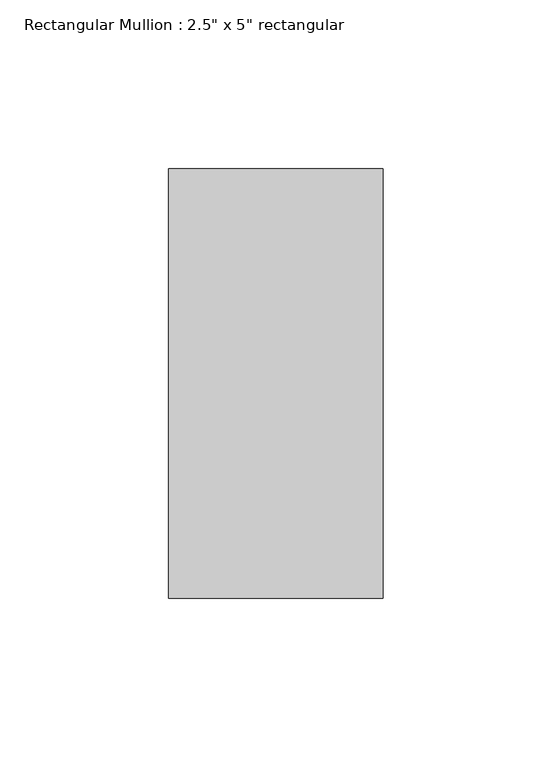
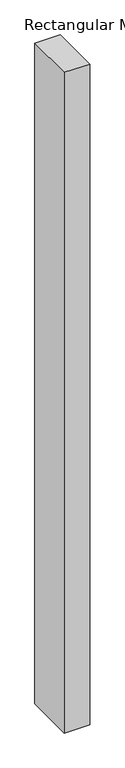
"""IFC4 building model written with IfcOpenShell, lengths in millimetres: member geometry."""

from ifc_helpers import new_model, si_unit, frame, origin, place, context, project, spatial, polyline, outline, extrude, source, transform, mapped, element, save


def member_93c3846a(model_context):
    return source(origin(), model_context, "Body", "SweptSolid", [
        extrude(outline(polyline([(31.75, 63.5), (31.75, -63.5), (-31.75, -63.5), (-31.75, 63.5), (31.75, 63.5)])), frame((0.0, 0.0, -1745.718644), z_axis=(0.0, 0.0, 1.0), x_axis=(1.0, 0.0, 0.0)), (0.0, 0.0, 1.0), 1745.718644),
    ])


if __name__ == "__main__":
    model = new_model("IFC4")
    model_context = context("Model", 3, world=origin())
    ifc_project = project(units=[si_unit("LENGTHUNIT", "METRE", prefix="MILLI")], contexts=[model_context])
    site = spatial("IfcSite", under=ifc_project)
    building = spatial("IfcBuilding", under=site)
    placement = place(None, origin())
    member_shape = member_93c3846a(model_context)
    element("IfcMember", 1, ObjectType="Rectangular Mullion : 2.5\" x 5\" rectangular", at=placement, inside=building, context=model_context, shape_type="MappedRepresentation", body=[
        mapped(member_shape, transform((0.0, 0.0, 0.0), x_axis=(1.0, 0.0, 0.0), y_axis=(0.0, 1.0, 0.0), z_axis=(0.0, 0.0, 1.0))),
    ])
    save(model, "model.ifc")

# Revit data of these elements
# Type "Rectangular Mullion : 2.5\" x 5\" rectangular"
#   built-in parameter 1007304 = 0.416667 (stored number, unit not read)
#   built-in parameter 1007301 = 0.104167 (stored number, unit not read)
#   built-in parameter 1007300 = 0.104167 (stored number, unit not read)
# Element 1 (IfcMember, "Rectangular Mullion : 2.5\" x 5\" rectangular")
#   Materials on its faces: "Aluminum"
# Materials
#   "Aluminum": class "Metal", colour RGB 247 247 247, transparency 0, Description = "Aluminum 6061", Cost = 0
